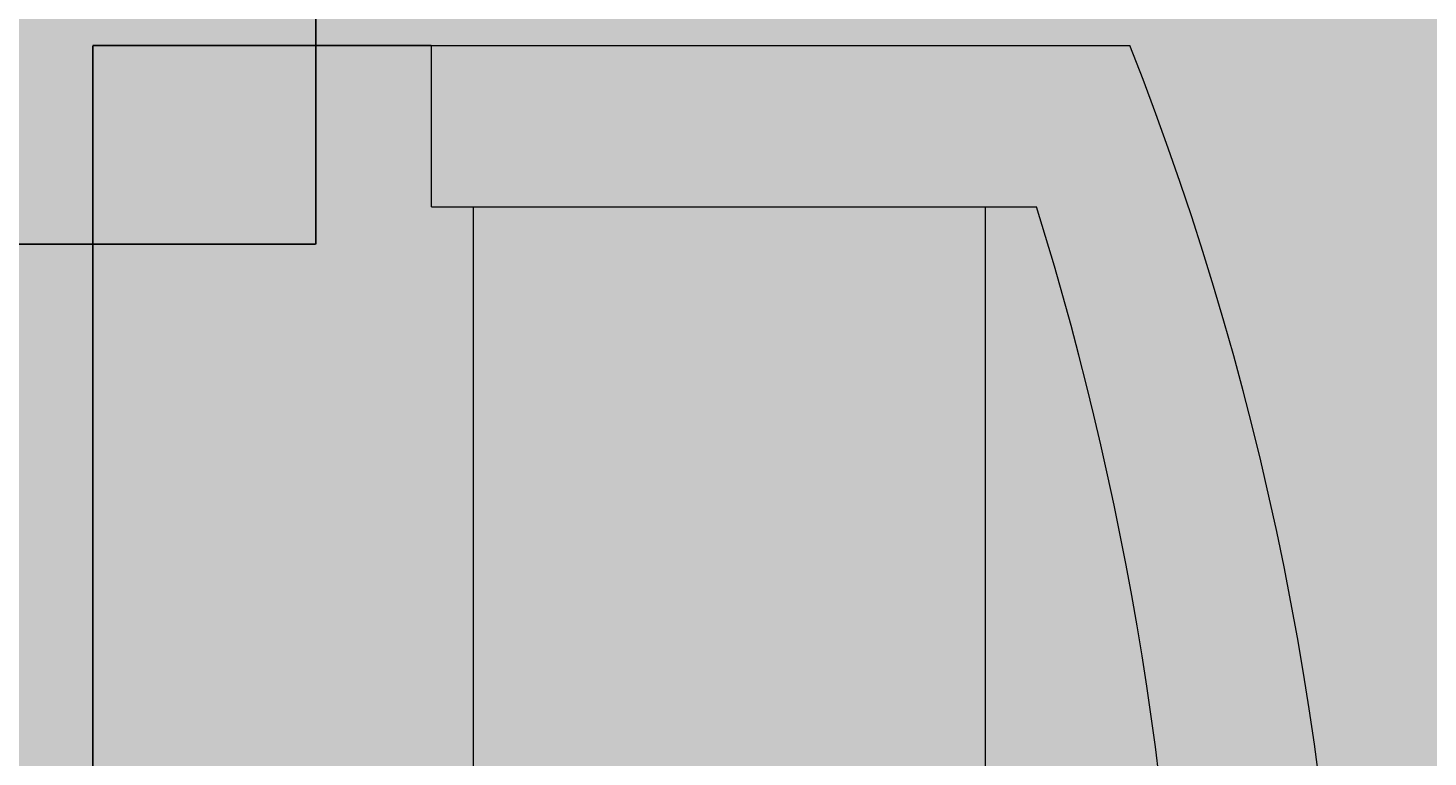
# Model space of a CAD drawing. Units: millimetres. Extents: x -229 to 16545, y -10488 to 4272.
# Tile 22 of 29: x 12629 to 13776, y -2708 to -2111. Entities that reach past the tile are written whole.
import ezdxf

# ---------------------------------------------------------------- set-up
doc = ezdxf.new("R2010")
doc.units = ezdxf.units.MM
for name, color, linetype, lineweight in [('A-ANNO-DIMS', 2, 'Continuous', 18), ('A-FURN', 8, 'Continuous', 18), ('A-FURN-PATT', 252, 'Continuous', 13)]:
    doc.layers.add(name, color=color, linetype=linetype, lineweight=lineweight)
doc.layers.add('A-FLOR-PATT', color=254, linetype='Continuous', lineweight=13, true_color=0xfeeab9)
doc.styles.get("Standard").update_dxf_attribs({"font": 'arial.ttf'})
doc.dimstyles.get("Standard").update_dxf_attribs({"dimtxt": 0.18, "dimasz": 0.18, "dimexe": 0.18, "dimexo": 0.0625, "dimgap": 0.09, "dimtad": 0, "dimtih": 1, "dimtoh": 1, "dimdec": 4, "dimzin": 0, "dimdsep": 46, "dimtxsty": 'Standard', "dimcen": 0.09, "dimadec": 0, "dimazin": 0, "dimtfac": 1, "dimtdec": 4, "dimtofl": 0, "dimtmove": 0, "dimatfit": 3, "dimfxl": 1, "dimtolj": 1, "dimtzin": 0, "dimarcsym": 0})

# ---------------------------------------------------------------- blocks, each defined once
blk = doc.blocks.new('Sofa - Roundback 7 ft.')
for p, q in [((-36.000027, -34), (-36.000027, -11.4696)), ((-35.999844, -13.3819), (35.9998, -13.3819)), ((-36.000027, -32.4421), (35.99998, -32.4421))]:
    blk.add_line(p, q)
blk.add_lwpolyline([(-36.000027, -34), (-42.000027, -34), (-42.000027, -8)])
for centre, radius, start, end in [((0, -114.25), 114.25, 68.43141, 111.5686), ((-0.00001, -127.1968), 121.1968, 72.72033, 107.2797)]:
    blk.add_arc(centre, radius, start, end)
blk = doc.blocks.new('*D37')
at = {"layer": 'A-ANNO-DIMS', "color": 0, "lineweight": -2, "transparency": 16777216}
for p, q in [((12959.5, -2125.1), (12682, -2125.1)), ((12682.2, -2125.3), (12682.2, -3049.5)), ((12682.2, -3974.1), (12682.2, -3049.9)), ((12959.5, -3974.3), (12682, -3974.3))]:
    blk.add_line(p, q, dxfattribs=at)
at = {"layer": 'A-ANNO-DIMS', "color": 0, "transparency": 16777216}
for points in [[(12682.2, -2125.3), (12682.2, -2125.3), (12682.2, -2125.1)], [(12682.2, -3974.1), (12682.2, -3974.1), (12682.2, -3974.3)]]:
    blk.add_solid(points, dxfattribs=at)
at = {"layer": 'Defpoints', "color": 0, "transparency": 16777216}
for p in [(12959.6, -2125.1), (12682.2, -3974.3), (12959.6, -3974.3)]:
    blk.add_point(p, dxfattribs=at)
at = {"layer": 'A-ANNO-DIMS', "color": 0, "transparency": 16777216, "insert": (12682.2, -3049.7), "char_height": 0.18, "attachment_point": 5}
blk.add_mtext('\\A1;SOFA 1849', dxfattribs=at)
blk = doc.blocks.new('*D39')
at = {"layer": 'A-ANNO-DIMS', "color": 0, "lineweight": -2, "transparency": 16777216}
for p, q in [((11588.8, -2096.3), (11588.8, -2287.9)), ((12864.9, -2096.3), (12864.9, -2287.9)), ((11588.9, -2287.7), (12225.8, -2287.7)), ((12864.7, -2287.7), (12227.9, -2287.7))]:
    blk.add_line(p, q, dxfattribs=at)
at = {"layer": 'A-ANNO-DIMS', "color": 0, "transparency": 16777216}
for points in [[(11588.9, -2287.7), (11588.9, -2287.7), (11588.8, -2287.7)], [(12864.7, -2287.7), (12864.7, -2287.7), (12864.9, -2287.7)]]:
    blk.add_solid(points, dxfattribs=at)
at = {"layer": 'Defpoints', "color": 0, "transparency": 16777216}
for p in [(11588.8, -2096.3), (12864.9, -2096.3), (12864.9, -2287.7)]:
    blk.add_point(p, dxfattribs=at)
at = {"layer": 'A-ANNO-DIMS', "color": 0, "transparency": 16777216, "insert": (12226.8, -2287.7), "char_height": 0.18, "attachment_point": 5}
blk.add_mtext('\\A1;LOVESEAT 1276', dxfattribs=at)

msp = doc.modelspace()

# ---------------------------------------------------------------- hatches: boundary and pattern name
at = {"layer": 'A-FLOR-PATT', "transparency": 33554592}
h = msp.add_hatch(color=256, dxfattribs=at)
h.dxf.hatch_style = 1
h.paths.add_polyline_path([(7975.933, -5325.772), (7943.121, -5325.772), (7943.121, -4576.49, 0.40145271), (7225.933, -5325.772, 0.40145271), (6508.746, -4576.49), (6508.746, -5325.772), (6475.933, -5325.772), (6475.933, -5438.272), (5975.933, -5438.272), (5975.933, -7267.724), (5975.933, -7438.272), (6478.619, -7438.272), (6463.448, -7355.919), (6464.88, -7356.837), (6463.849, -7358.097), (6478.619, -7438.272), (6610.327, -7438.272), (6632.656, -7409.564), (6632.525, -7406.967), (6634.208, -7407.569), (6619.273, -7426.77), (6654.466, -7438.272), (7610.517, -7438.272), (7607.41, -7421.409), (7608.842, -7422.327), (7607.812, -7423.587), (7610.517, -7438.272), (7975.933, -7438.272)])
h.paths.add_polyline_path([(13785.933, -1208.272), (9555.933, -1208.272), (9555.933, -961.785), (9705.933, -961.785), (9705.933, -918.035), (10704.976, -918.035, 0.40145271), (9705.933, 38.215), (9555.933, 38.215), (9555.933, 2021.728), (5975.933, 2021.728), (5975.933, 755.492), (5745.933, 755.492), (5745.933, 1427.266), (2918.813, 1427.266), (2918.813, -492.942), (5013.319, -492.942), (5013.319, -978.272), (5745.933, -978.272), (5745.933, -397.513), (5975.933, -397.513), (5975.933, -1208.272), (4560.933, -1208.272), (4560.933, -1265.772), (4448.433, -1265.772), (4448.433, -1298.585), (4445.933, -1298.585), (3699.151, -1298.585, 0.40145271), (4448.433, -2015.772), (4560.933, -2015.772), (4560.933, -2384.177), (5745.933, -2384.177), (5799.402, -2384.177), (5799.402, -4518.272), (5975.933, -4518.272), (5975.933, -5208.272), (6475.933, -5208.272), (6475.933, -4575.772), (6508.746, -4575.772), (6508.746, -4576.49, -0.35647263), (7216.672, -5208.272), (7235.194, -5208.272, -0.35647263), (7943.121, -4576.49), (7943.121, -4575.772), (7975.933, -4575.772), (7975.933, -5208.272), (11176.247, -5208.272), (11159.44, -5191.465), (10520.768, -5191.465), (10520.768, -4888.936), (10571.19, -4888.936), (10571.19, -4872.129), (10772.876, -4872.129), (10772.876, -4888.936), (10789.683, -4888.936), (10789.683, -4872.129), (10991.368, -4872.129), (10991.368, -4888.936), (11041.79, -4888.936), (11041.79, -4872.129), (11058.597, -4872.129, -0.09090909), (11428.354, -4872.129), (11445.162, -4872.129), (11445.162, -4888.936), (11529.197, -4888.936), (11529.197, -5191.465), (11327.512, -5191.465), (11310.704, -5208.272), (13785.933, -5208.272)])
h.paths.add_polyline_path([(11047.216, -1630.944, -1), (11402.816, -1630.944, -1)], flags=16)
h.paths.add_polyline_path([(11148.816, -1630.944), (11225.016, -1554.744), (11301.216, -1630.944), (11225.016, -1707.144)], flags=0)
h.paths.add_polyline_path([(11199.616, -1630.944, -1), (11250.416, -1630.944, -1)], flags=0)
h.paths.add_polyline_path([(11588.751, -2096.259), (11588.751, -1543.254, -0.26666697), (12864.918, -1543.254), (12864.918, -2096.259), (12737.302, -2096.259), (12737.302, -2063.121), (11716.368, -2063.121), (11716.368, -2096.259)], flags=16)
h.paths.add_polyline_path([(12012.696, -2489.42), (12600.997, -2489.42), (12600.997, -3666.022), (12012.696, -3666.022)], flags=16)
h.paths.add_polyline_path([(12176.41, -3599.403), (12174.938, -3609.076), (12173.789, -3618.819), (12173.09, -3628.559), (12172.973, -3638.221), (12173.89, -3652.852), (12175.008, -3657.025), (12172.909, -3643.473), (12173.142, -3624.297), (12175.386, -3605.273)], flags=0)
h.paths.add_polyline_path([(8026.289, -286.944), (7737.703, -287.19), (7734.87, -269.156), (8029.092, -268.905)], flags=16)
h.paths.add_polyline_path([(7733.453, -260.139), (7710.784, -115.865), (7557.191, -115.996), (7556.999, 109.744), (7412.687, 132.166), (7412.433, 429.206), (7556.707, 451.876), (7556.568, 614.769), (7412.256, 637.19), (7412.003, 934.231), (7556.276, 956.9), (7556.084, 1182.639), (7709.677, 1182.77), (7732.099, 1327.082), (8029.14, 1327.335), (8051.808, 1183.062), (8205.401, 1183.192), (8205.594, 957.454), (8349.906, 935.031), (8350.159, 637.99), (8205.885, 615.322), (8206.024, 452.43), (8350.336, 430.006), (8350.59, 132.965), (8206.316, 110.298), (8206.509, -115.442), (8052.916, -115.573), (8030.493, -259.885)], flags=16)
h.paths.add_polyline_path([(12261.416, -3475.554), (12262.632, -3486.776), (12264.032, -3497.007), (12265.554, -3506.365), (12267.136, -3514.968), (12268.719, -3522.935), (12271.304, -3535.59), (12273.606, -3548.078), (12275.271, -3561.064), (12275.93, -3574.938), (12275.325, -3590.3), (12273.425, -3607.964), (12270.795, -3625.658), (12268.066, -3641.063), (12266.318, -3649.679), (12265.456, -3653.626), (12263.984, -3659.846), (12264.032, -3659.566), (12264.342, -3658.241), (12264.807, -3656.37), (12265.456, -3653.626), (12266.318, -3649.679), (12267.409, -3644.302), (12268.668, -3637.664), (12270.019, -3630.037), (12271.384, -3621.695), (12272.69, -3612.908), (12273.857, -3603.948), (12274.81, -3595.088), (12275.47, -3586.601), (12275.782, -3578.689), (12275.757, -3571.292), (12275.423, -3564.275), (12274.816, -3557.512), (12273.964, -3550.872), (12272.896, -3544.224), (12271.645, -3537.439), (12270.24, -3530.385), (12267.543, -3517.181), (12264.612, -3501.247), (12261.849, -3481.059)], flags=0)
h.paths.add_polyline_path([(12332.136, -3408.03), (12333.483, -3416.79), (12335.077, -3424.54), (12336.915, -3431.355), (12338.991, -3437.32), (12341.266, -3442.55), (12343.694, -3447.166), (12346.229, -3451.292), (12348.826, -3455.051), (12351.438, -3458.563), (12357.476, -3466.491), (12363.61, -3476.575), (12368.309, -3489.762), (12369.929, -3503.427), (12369.842, -3516.511), (12368.43, -3530.867), (12365.816, -3545.835), (12362.382, -3559.786), (12360.968, -3564.487), (12363.063, -3557.021), (12364.898, -3549.566), (12366.473, -3542.077), (12367.773, -3534.631), (12368.781, -3527.301), (12369.483, -3520.162), (12369.863, -3513.291), (12369.906, -3506.759), (12369.599, -3500.643), (12368.93, -3494.999), (12367.924, -3489.796), (12366.61, -3484.994), (12365.024, -3480.542), (12363.19, -3476.399), (12361.141, -3472.516), (12358.909, -3468.847), (12356.525, -3465.347), (12354.02, -3461.954), (12351.438, -3458.563), (12345.462, -3450.529), (12339.923, -3439.996), (12335.85, -3428.296), (12332.68, -3412.888)], flags=0)
h.paths.add_polyline_path([(12385.287, -3334.612), (12384.977, -3342.409), (12385.02, -3349.196), (12385.4, -3355.066), (12386.104, -3360.105), (12387.112, -3364.41), (12388.412, -3368.071), (12389.987, -3371.181), (12391.823, -3373.832), (12393.919, -3376.097), (12396.337, -3377.978), (12399.153, -3379.462), (12402.445, -3380.531), (12406.289, -3381.172), (12410.758, -3381.371), (12415.935, -3381.106), (12421.893, -3380.368), (12428.658, -3379.159), (12436.069, -3377.55), (12443.907, -3375.635), (12451.961, -3373.505), (12460.015, -3371.254), (12467.853, -3368.971), (12475.263, -3366.749), (12482.029, -3364.68), (12491.877, -3361.657), (12497.701, -3360.107), (12501.639, -3359.288), (12510.135, -3358.326), (12519.662, -3365.412), (12524.243, -3378.911), (12523.764, -3390.7), (12520.746, -3401.577), (12514.248, -3415.634), (12511.518, -3420.418), (12515.856, -3412.154), (12519.153, -3405.024), (12521.516, -3398.804), (12523.049, -3393.276), (12523.865, -3388.212), (12524.059, -3383.441), (12523.7, -3378.958), (12522.853, -3374.815), (12521.576, -3371.054), (12519.931, -3367.722), (12517.982, -3364.865), (12515.786, -3362.529), (12513.405, -3360.758), (12510.877, -3359.588), (12508.136, -3358.982), (12505.086, -3358.897), (12501.639, -3359.288), (12497.701, -3360.107), (12493.183, -3361.309), (12487.988, -3362.851), (12476.403, -3366.408), (12463.335, -3370.326), (12447.372, -3374.788), (12431.759, -3378.604), (12418.504, -3380.974), (12405.811, -3381.624), (12394.725, -3378.025), (12388.039, -3368.367), (12385.583, -3357.877), (12384.826, -3346.204), (12385.428, -3331.059), (12385.953, -3325.719)], flags=0)
h.paths.add_polyline_path([(7880.016, 1173.969), (7880.373, 1175.495), (7880.433, 1175.851), (7879.484, 1171.818)], flags=0)
h.paths.add_polyline_path([(7802.33, 874.962), (7800.771, 885.032), (7798.932, 893.941), (7796.811, 901.774), (7794.419, 908.63), (7791.798, 914.639), (7789.002, 919.945), (7786.083, 924.686), (7783.093, 929.005), (7780.087, 933.043), (7774.996, 939.717), (7768.406, 949.37), (7762.174, 963.427), (7759.342, 978.002), (7758.629, 991.888), (7759.492, 1007.928), (7761.801, 1025.496), (7765.392, 1044.035), (7766.625, 1049.048), (7764.522, 1039.543), (7762.719, 1030.232), (7761.232, 1021.168), (7760.08, 1012.405), (7759.28, 1003.994), (7758.849, 995.988), (7758.806, 988.44), (7759.167, 981.404), (7759.942, 974.914), (7761.104, 968.936), (7762.617, 963.414), (7764.448, 958.299), (7766.559, 953.535), (7768.918, 949.073), (7771.487, 944.856), (7774.232, 940.835), (7777.115, 936.938), (7782.377, 930.041), (7787.845, 922.139), (7793.348, 911.698), (7798.042, 898.247), (7801.702, 880.527)], flags=0)
h.paths.add_polyline_path([(12519.068, -3228.534), (12519.615, -3236.235), (12520.529, -3242.343), (12521.78, -3247.103), (12523.337, -3250.758), (12525.171, -3253.556), (12527.248, -3255.709), (12529.522, -3257.296), (12531.95, -3258.361), (12534.486, -3258.949), (12537.082, -3259.11), (12539.694, -3258.888), (12542.277, -3258.329), (12544.781, -3257.478), (12547.173, -3256.388), (12549.46, -3255.129), (12550.455, -3254.517), (12555.825, -3251.109), (12557.835, -3249.942), (12565.181, -3246.404), (12574.565, -3253.032), (12576.931, -3265.022), (12576.627, -3277.425), (12575.416, -3290.819), (12574.851, -3295.392), (12575.708, -3287.593), (12576.322, -3280.806), (12576.688, -3274.939), (12576.812, -3269.899), (12576.688, -3265.593), (12576.322, -3261.932), (12575.708, -3258.822), (12574.851, -3256.172), (12573.753, -3253.905), (12572.439, -3252.005), (12570.943, -3250.474), (12569.293, -3249.309), (12567.523, -3248.513), (12565.658, -3248.083), (12563.732, -3248.022), (12561.777, -3248.328), (12559.814, -3248.989), (12557.835, -3249.942), (12555.825, -3251.109), (12553.77, -3252.413), (12551.652, -3253.78), (12549.46, -3255.129), (12543.167, -3258.594), (12532.661, -3259.485), (12524.685, -3253.923), (12520.949, -3245.152), (12519.138, -3233.042)], flags=0)
h.paths.add_polyline_path([(7741.293, 790.501), (7741.641, 799.467), (7741.584, 807.269), (7741.141, 814.015), (7740.329, 819.809), (7739.165, 824.757), (7737.667, 828.966), (7735.853, 832.541), (7733.74, 835.586), (7731.348, 838.188), (7728.71, 840.348), (7725.861, 842.052), (7722.836, 843.28), (7719.671, 844.015), (7716.4, 844.237), (7713.06, 843.932), (7709.684, 843.081), (7706.304, 841.686), (7702.923, 839.834), (7699.543, 837.629), (7696.164, 835.178), (7692.784, 832.585), (7684.718, 826.315), (7675.609, 820.63), (7664.001, 817.274), (7654.105, 821.884), (7647.171, 832.02), (7644.191, 846.522), (7646.321, 860.288), (7647.49, 864.223), (7645.946, 857.865), (7645.046, 852.044), (7644.827, 846.557), (7645.243, 841.404), (7646.221, 836.642), (7647.693, 832.318), (7649.587, 828.489), (7651.832, 825.206), (7654.359, 822.523), (7657.097, 820.49), (7659.984, 819.145), (7662.993, 818.452), (7666.108, 818.357), (7669.311, 818.809), (7672.583, 819.755), (7675.908, 821.139), (7679.268, 822.913), (7682.645, 825.021), (7686.025, 827.401), (7689.404, 829.958), (7692.784, 832.585), (7700.505, 838.509), (7709.871, 843.64), (7721.436, 844.698), (7733.277, 837.617), (7739.571, 825.214), (7741.557, 811.049), (7741.669, 795.575)], flags=0)
h.paths.add_polyline_path([(8377.641, 137.216), (8359.607, 134.382), (8359.356, 428.605), (8377.395, 425.802)], flags=16)
h.paths.add_polyline_path([(7650.715, 668.465), (7650.08, 677.319), (7649.023, 684.34), (7647.579, 689.811), (7645.785, 694.012), (7643.675, 697.228), (7641.286, 699.7), (7638.669, 701.521), (7635.876, 702.744), (7632.96, 703.419), (7629.974, 703.601), (7626.971, 703.344), (7624.004, 702.697), (7621.125, 701.717), (7618.375, 700.462), (7615.749, 699.013), (7614.561, 698.279), (7608.435, 694.382), (7606.125, 693.04), (7598.981, 689.594), (7589.669, 693.773), (7585.26, 702.856), (7584.221, 713.11), (7584.49, 724.584), (7585.863, 739.937), (7586.518, 745.277), (7585.539, 736.31), (7584.841, 728.507), (7584.424, 721.761), (7584.288, 715.966), (7584.433, 711.016), (7584.86, 706.807), (7585.567, 703.231), (7586.556, 700.186), (7587.821, 697.58), (7589.332, 695.397), (7591.053, 693.637), (7592.951, 692.3), (7594.989, 691.385), (7597.132, 690.895), (7599.346, 690.826), (7601.594, 691.18), (7603.851, 691.943), (7606.125, 693.04), (7608.435, 694.382), (7610.797, 695.885), (7613.229, 697.458), (7620.475, 701.929), (7632.001, 704.44), (7643.476, 699.417), (7648.536, 687.571), (7650.63, 673.661)], flags=0)
h.paths.add_polyline_path([(7385.628, 136.37), (7385.382, 424.956), (7403.416, 427.789), (7403.667, 133.567)], flags=16)
h.paths.add_polyline_path([(12993.884, -2257.186), (12959.588, -2257.186), (12959.588, -2125.099), (13531.966, -2125.099, -0.19047621), (13531.966, -3974.321), (12959.588, -3974.321), (12959.588, -3842.233), (12993.884, -3842.233)], flags=16)
h.paths.add_polyline_path([(13413.486, -3313.884), (13413.486, -2785.535), (13562.885, -2785.535, -0.04962821), (13562.885, -3313.884)], flags=0)
h.paths.add_polyline_path([(8377.21, 642.241), (8359.176, 639.407), (8358.925, 933.629), (8376.964, 930.826)], flags=16)
h.paths.add_polyline_path([(13086.058, -1864.83), (13086.058, -1449.84), (13501.048, -1449.84), (13501.048, -1864.83)], flags=16)
h.paths.add_polyline_path([(13305.814, -1862.197), (13302.103, -1859.624), (13298.088, -1857.068), (13293.799, -1854.536), (13289.262, -1852.031), (13284.504, -1849.559), (13279.554, -1847.125), (13274.439, -1844.735), (13269.17, -1842.389), (13263.701, -1840.081), (13257.97, -1837.797), (13251.914, -1835.525), (13245.472, -1833.252), (13238.582, -1830.968), (13231.18, -1828.66), (13223.206, -1826.315), (13209.182, -1822.458), (13204.584, -1821.48), (13217.962, -1824.773), (13235.072, -1829.804), (13248.777, -1834.349), (13260.829, -1838.869), (13274.479, -1844.63), (13289.675, -1852.101), (13302.553, -1859.704)], flags=0)
h.paths.add_polyline_path([(13428.104, -1820.994), (13419.007, -1818.141), (13409.95, -1815.4), (13400.766, -1812.747), (13391.271, -1810.151), (13376.087, -1806.251), (13370.618, -1805.019), (13386.304, -1808.794), (13405.087, -1813.928), (13423.014, -1819.354)], flags=0)
h.paths.add_polyline_path([(7385.197, 641.395), (7384.951, 929.98), (7402.986, 932.814), (7403.236, 638.592)], flags=16)
h.paths.add_polyline_path([(13262.537, -1725.526), (13253.246, -1724.74), (13244.516, -1724.117), (13235.94, -1723.625), (13223.267, -1723.062), (13217.598, -1722.912), (13231.966, -1723.397), (13248.733, -1724.359), (13266.899, -1725.895), (13272.802, -1726.502)], flags=0)
h.paths.add_polyline_path([(13191.893, -1641.137), (13208.675, -1640.506), (13214.057, -1640.258), (13197.763, -1640.936)], flags=0)
h.paths.add_polyline_path([(13097.524, -1608.457), (13114.284, -1609.031), (13120.126, -1609.105), (13103.045, -1608.71)], flags=0)
h.paths.add_polyline_path([(13465.328, -1521.577), (13473.906, -1517.015), (13481.761, -1511.636), (13492.562, -1502.076), (13495.327, -1497.933), (13485.818, -1508.858), (13470.208, -1519.547)], flags=0)
h.paths.add_polyline_path([(13175.015, -1500.891), (13184.046, -1501.807), (13192.721, -1502.52), (13201.114, -1503.034), (13209.273, -1503.351), (13217.244, -1503.476), (13225.078, -1503.41), (13232.821, -1503.16), (13240.524, -1502.728), (13248.233, -1502.117), (13255.993, -1501.322), (13263.825, -1500.293), (13271.746, -1498.974), (13279.775, -1497.305), (13287.928, -1495.229), (13296.222, -1492.688), (13304.675, -1489.622), (13313.304, -1485.975), (13322.089, -1481.727), (13330.859, -1477.028), (13339.408, -1472.063), (13347.526, -1467.02), (13355.006, -1462.087), (13364.86, -1455.202), (13367.224, -1453.299), (13358.544, -1459.754), (13343.348, -1469.775), (13326.143, -1479.767), (13309.023, -1488.045), (13292.249, -1494.129), (13276.009, -1498.264), (13260.299, -1500.88), (13244.401, -1502.51), (13228.945, -1503.378), (13213.316, -1503.508), (13197.047, -1502.876), (13180.088, -1501.481)], flags=0)
h.paths.add_polyline_path([(7733.501, 1336.101), (7736.303, 1354.14), (8024.889, 1354.386), (8027.723, 1336.352)], flags=16)
at = {"layer": 'A-FURN-PATT'}
h = msp.add_hatch(color=256, dxfattribs=at)
h.dxf.hatch_style = 1
h.paths.add_polyline_path([(13413.486, -2257.186), (12993.884, -2257.186), (12993.884, -2785.535), (13413.486, -2785.535)], flags=17)
h.paths.add_polyline_path([(13413.486, -2785.535), (12993.884, -2785.535), (12993.884, -3313.884), (13413.486, -3313.884)], flags=17)
h.paths.add_polyline_path([(13413.486, -3313.884), (12993.884, -3313.884), (12993.884, -3842.233), (13413.486, -3842.233)], flags=17)
h.paths.add_polyline_path([(13531.966, -2125.099), (12959.588, -2125.099), (12959.588, -2257.186), (13455.573, -2257.186, -0.15194781), (13455.573, -3842.233), (12959.588, -3842.233), (12959.588, -3974.321), (13531.966, -3974.321, 0.19047621)])
h.paths.add_polyline_path([(13455.573, -2257.186), (13413.486, -2257.186), (13413.486, -2785.535), (13562.885, -2785.535, 0.05064665)], flags=17)
h.paths.add_polyline_path([(13562.885, -2785.535), (13413.486, -2785.535), (13413.486, -3313.884), (13562.885, -3313.884, 0.04962821)], flags=17)
h.paths.add_polyline_path([(13562.885, -3313.884), (13413.486, -3313.884), (13413.486, -3842.233), (13455.573, -3842.233, 0.05064665)], flags=17)
h.paths.add_polyline_path([(11588.751, -1543.254), (11588.751, -2096.259), (11716.368, -2096.259), (11716.368, -1617.061, -0.22792319), (12737.302, -1617.061), (12737.302, -2096.259), (12864.918, -2096.259), (12864.918, -1543.254, 0.26666697)])
h.paths.add_polyline_path([(12226.834, -1500.713, 0.11251869), (11716.368, -1617.061), (11716.368, -1657.721), (12226.834, -1657.721)], flags=17)
h.paths.add_polyline_path([(12737.302, -1617.061, 0.11251889), (12226.834, -1500.713), (12226.834, -1657.721), (12737.302, -1657.721)], flags=17)
h.paths.add_polyline_path([(12226.834, -1657.721), (11716.368, -1657.721), (11716.368, -2063.121), (12226.834, -2063.121)], flags=17)
h.paths.add_polyline_path([(12737.302, -1657.721), (12226.834, -1657.721), (12226.834, -2063.121), (12737.302, -2063.121)], flags=17)

# ---------------------------------------------------------------- block references
at = {"layer": 'A-FURN', "xscale": 22.01454356165477, "yscale": 22.01454356165477, "zscale": 22.01454356165477, "rotation": 270}
msp.add_blockref('Sofa - Roundback 7 ft.', (13708.082, -3049.71), dxfattribs=at)

# ---------------------------------------------------------------- dimensions: what is measured, and where the dimension line sits
at = {"layer": 'A-ANNO-DIMS'}
dim = msp.add_linear_dim(base=(12864.918, -2287.684), p1=(11588.751, -2096.259), p2=(12864.918, -2096.259), text='LOVESEAT <>', dimstyle='Standard', override={"dimdec": 0, "dimlfac": 1, "dimrnd": 0, "dimzin": 0, "dimdsep": 46, "dimlunit": 2}, dxfattribs=at)
dim.commit()
dim.dimension.update_dxf_attribs({"geometry": '*D39', "text_midpoint": (12226.835, -2287.684)})
dim = msp.add_linear_dim(base=(12682.205, -3974.321), p1=(12959.588, -2125.099), p2=(12959.588, -3974.321), angle=270, text='SOFA <>', dimstyle='Standard', override={"dimdec": 0, "dimlfac": 1, "dimrnd": 0, "dimzin": 0, "dimdsep": 46, "dimlunit": 2}, dxfattribs=at)
dim.commit()
dim.dimension.update_dxf_attribs({"geometry": '*D37', "text_midpoint": (12682.205, -3049.71)})

doc.saveas('drawing.dxf')
